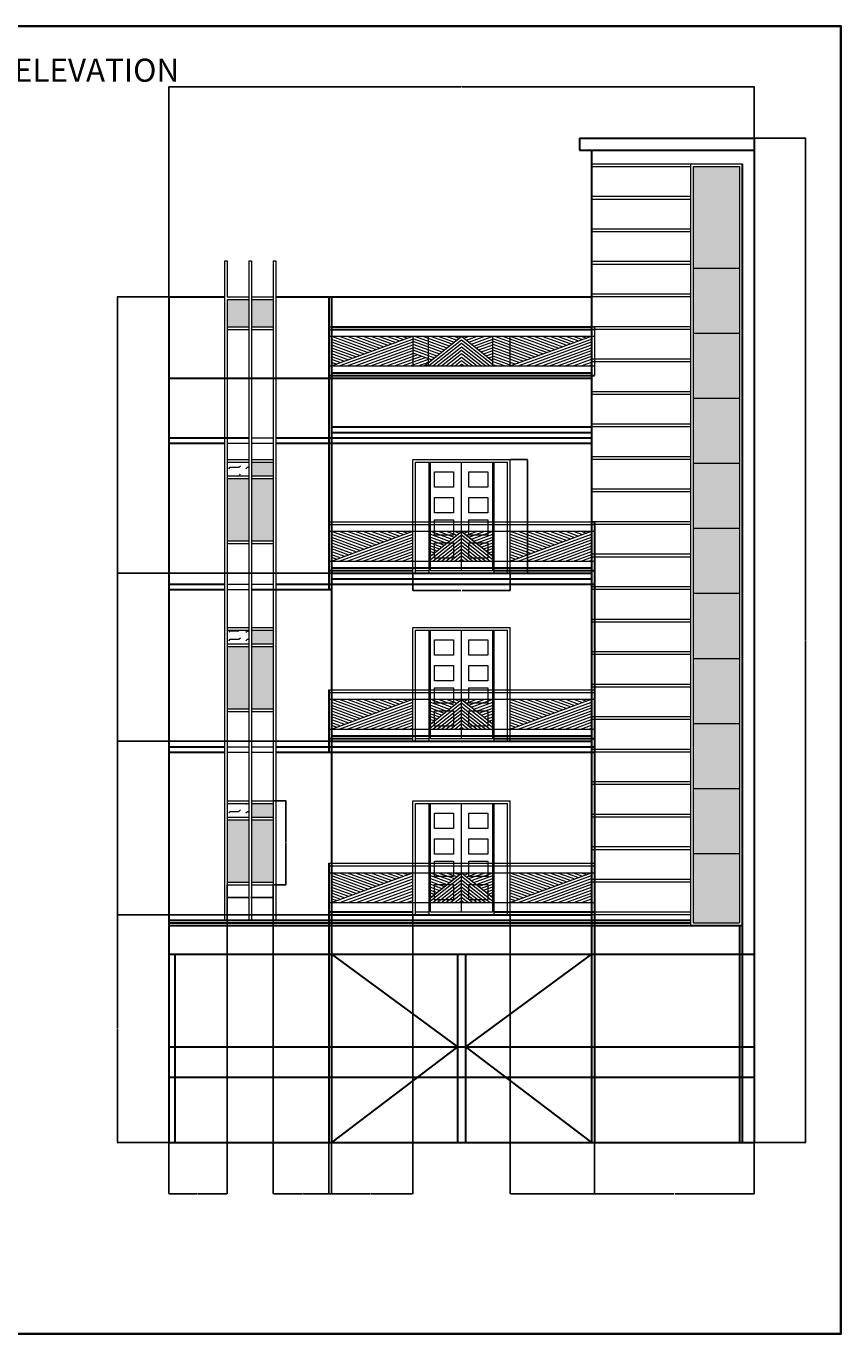
# Model space of a CAD drawing. Units: inches. Extents: x 2220 to 3422, y 783 to 1748.
# Tile 7 of 7: x 2821 to 3422, y 783 to 1748. Entities that reach past the tile are written whole.
import ezdxf

# ---------------------------------------------------------------- set-up
doc = ezdxf.new("R2010")
doc.units = ezdxf.units.IN
for name, color, linetype, lineweight in [('A-ANNO-DIMS', 2, 'Continuous', 18), ('A-ANNO-TEXT', 7, 'Continuous', 30), ('A-ANNO-TTLB', 7, 'Continuous', 35), ('A-ELEV', 7, 'Continuous', 30), ('A-ELEV-CLAD', 8, 'Continuous', 18), ('A-ELEV-DOOR', 3, 'Continuous', 20), ('A-ELEV-GLAZ', 4, 'Continuous', 18), ('A-ELEV-PATT', 252, 'Continuous', 13), ('A-ELEV-RAIL', 7, 'Continuous', 20)]:
    doc.layers.add(name, color=color, linetype=linetype, lineweight=lineweight)
doc.styles.get("Standard").update_dxf_attribs({"font": 'arial.ttf'})
doc.dimstyles.get("Standard").update_dxf_attribs({"dimtxt": 0.18, "dimasz": 0.18, "dimexe": 0.18, "dimexo": 0.0625, "dimgap": 0.09, "dimtad": 0, "dimtih": 1, "dimtoh": 1, "dimdec": 4, "dimzin": 0, "dimdsep": 46, "dimtxsty": 'Standard', "dimcen": 0.09, "dimadec": 0, "dimazin": 0, "dimtfac": 1, "dimtdec": 4, "dimtofl": 0, "dimtmove": 0, "dimatfit": 3, "dimfxl": 1, "dimtolj": 1, "dimtzin": 0, "dimarcsym": 0})

# ---------------------------------------------------------------- blocks, each defined once
blk = doc.blocks.new('DOOR-ELEV-DOUBLE-PANELED')
for p, q in [((0, 0), (0, 84)), ((0, 84), (72, 84)), ((2, 0), (2, 82)), ((2, 82), (70, 82)), ((12, 0), (12, 82)), ((13, 2), (13, 82)), ((36, 2), (36, 82)), ((59, 2), (59, 82)), ((60, 0), (60, 82)), ((70, 0), (70, 82)), ((72, 0), (72, 84)), ((2, 2), (12, 2)), ((13, 2), (59, 2))]:
    blk.add_line(p, q)
for points in [[(16.01, 74.85), (30.01, 74.85), (30.01, 63.54), (16.01, 63.54)], [(41.44, 74.85), (55.44, 74.85), (55.44, 63.54), (41.44, 63.54)], [(16.01, 55.98), (30.01, 55.98), (30.01, 44.68), (16.01, 44.68)], [(41.44, 55.98), (55.44, 55.98), (55.44, 44.68), (41.44, 44.68)], [(16.01, 39.54), (30.01, 39.54), (30.01, 28.24), (16.01, 28.24)], [(41.44, 39.54), (55.44, 39.54), (55.44, 28.24), (41.44, 28.24)], [(16.01, 22.35), (30.01, 22.35), (30.01, 11.05), (16.01, 11.05)], [(41.44, 22.35), (55.44, 22.35), (55.44, 11.05), (41.44, 11.05)]]:
    blk.add_lwpolyline(points, close=True)
blk = doc.blocks.new('GLAZ-ELEV-PAIRED-LIGHTS')
for p, q in [((0, 62), (16, 62)), ((0, 60), (16, 60)), ((0, 60), (0, 50)), ((18, 62), (34, 62)), ((18, 60), (34, 60)), ((34, 60), (34, 50)), ((0, 50), (16, 50)), ((18, 50), (34, 50)), ((0, 48), (16, 48)), ((0, 48), (0, 2)), ((18, 48), (34, 48)), ((34, 48), (34, 2)), ((0, 2), (16, 2)), ((0, 0), (16, 0)), ((18, 2), (34, 2)), ((18, 0), (34, 0))]:
    blk.add_line(p, q)
blk = doc.blocks.new('*D33')
at = {"layer": 'A-ANNO-DIMS', "color": 0, "lineweight": -2, "transparency": 16777216}
for p, q in [((3178.51, 1428.15), (3191.23, 1428.15)), ((3191.05, 1427.97), (3191.05, 1386.33)), ((3191.05, 1344.33), (3191.05, 1385.97)), ((3178.51, 1344.15), (3191.23, 1344.15))]:
    blk.add_line(p, q, dxfattribs=at)
at = {"layer": 'A-ANNO-DIMS', "color": 0, "transparency": 16777216}
for points in [[(3191.02, 1427.97), (3191.08, 1427.97), (3191.05, 1428.15)], [(3191.02, 1344.33), (3191.08, 1344.33), (3191.05, 1344.15)]]:
    blk.add_solid(points, dxfattribs=at)
at = {"layer": 'Defpoints', "color": 0, "transparency": 16777216}
for p in [(3178.45, 1428.15), (3191.05, 1428.15), (3178.45, 1344.15)]:
    blk.add_point(p, dxfattribs=at)
at = {"layer": 'A-ANNO-DIMS', "color": 0, "transparency": 16777216, "insert": (3191.05, 1386.15), "char_height": 0.18, "attachment_point": 5}
blk.add_mtext('\\A1;DOUBLE DOOR 84 TYP.', dxfattribs=at)
blk = doc.blocks.new('*D34')
at = {"layer": 'A-ANNO-DIMS', "color": 0, "lineweight": -2, "transparency": 16777216}
for p, q in [((3106.45, 1344.09), (3106.45, 1331.37)), ((3178.45, 1344.09), (3178.45, 1331.37)), ((3106.63, 1331.55), (3141.92, 1331.55)), ((3178.27, 1331.55), (3142.97, 1331.55))]:
    blk.add_line(p, q, dxfattribs=at)
at = {"layer": 'A-ANNO-DIMS', "color": 0, "transparency": 16777216}
for points in [[(3106.63, 1331.58), (3106.63, 1331.52), (3106.45, 1331.55)], [(3178.27, 1331.58), (3178.27, 1331.52), (3178.45, 1331.55)]]:
    blk.add_solid(points, dxfattribs=at)
at = {"layer": 'Defpoints', "color": 0, "transparency": 16777216}
for p in [(3106.45, 1344.15), (3178.45, 1344.15), (3178.45, 1331.55)]:
    blk.add_point(p, dxfattribs=at)
at = {"layer": 'A-ANNO-DIMS', "color": 0, "transparency": 16777216, "insert": (3142.45, 1331.55), "char_height": 0.18, "attachment_point": 5}
blk.add_mtext('\\A1;72 TYP.', dxfattribs=at)
blk = doc.blocks.new('*D35')
at = {"layer": 'A-ANNO-DIMS', "color": 0, "lineweight": -2, "transparency": 16777216}
for p, q in [((3003.51, 1176.15), (3012.93, 1176.15)), ((3012.75, 1175.97), (3012.75, 1145.33)), ((3012.75, 1114.33), (3012.75, 1144.97)), ((3003.51, 1114.15), (3012.93, 1114.15))]:
    blk.add_line(p, q, dxfattribs=at)
at = {"layer": 'A-ANNO-DIMS', "color": 0, "transparency": 16777216}
for points in [[(3012.72, 1175.97), (3012.78, 1175.97), (3012.75, 1176.15)], [(3012.72, 1114.33), (3012.78, 1114.33), (3012.75, 1114.15)]]:
    blk.add_solid(points, dxfattribs=at)
at = {"layer": 'Defpoints', "color": 0, "transparency": 16777216}
for p in [(3003.45, 1176.15), (3012.75, 1176.15), (3003.45, 1114.15)]:
    blk.add_point(p, dxfattribs=at)
at = {"layer": 'A-ANNO-DIMS', "color": 0, "transparency": 16777216, "insert": (3012.75, 1145.15), "char_height": 0.18, "attachment_point": 5}
blk.add_mtext('\\A1;PAIRED LIGHTS 62 TYP.', dxfattribs=at)
blk = doc.blocks.new('*D36')
at = {"layer": 'A-ANNO-DIMS', "color": 0, "lineweight": -2, "transparency": 16777216}
for p, q in [((2969.45, 1114.09), (2969.45, 1104.67)), ((3003.45, 1114.09), (3003.45, 1104.67)), ((2969.63, 1104.85), (2985.92, 1104.85)), ((3003.27, 1104.85), (2986.97, 1104.85))]:
    blk.add_line(p, q, dxfattribs=at)
at = {"layer": 'A-ANNO-DIMS', "color": 0, "transparency": 16777216}
for points in [[(2969.63, 1104.88), (2969.63, 1104.82), (2969.45, 1104.85)], [(3003.27, 1104.88), (3003.27, 1104.82), (3003.45, 1104.85)]]:
    blk.add_solid(points, dxfattribs=at)
at = {"layer": 'Defpoints', "color": 0, "transparency": 16777216}
for p in [(2969.45, 1114.15), (3003.45, 1114.15), (3003.45, 1104.85)]:
    blk.add_point(p, dxfattribs=at)
at = {"layer": 'A-ANNO-DIMS', "color": 0, "transparency": 16777216, "insert": (2986.45, 1104.85), "char_height": 0.18, "attachment_point": 5}
blk.add_mtext('\\A1;34 TYP.', dxfattribs=at)
blk = doc.blocks.new('*D61')
at = {"layer": 'A-ANNO-DIMS', "color": 0, "lineweight": -2, "transparency": 16777216}
for p, q in [((2926.45, 1548.21), (2926.45, 1703.46)), ((2926.63, 1703.28), (3142.15, 1703.28)), ((3358.27, 1703.28), (3142.74, 1703.28)), ((3358.45, 1665.44), (3358.45, 1703.46))]:
    blk.add_line(p, q, dxfattribs=at)
at = {"layer": 'A-ANNO-DIMS', "color": 0, "transparency": 16777216}
for points in [[(2926.63, 1703.31), (2926.63, 1703.25), (2926.45, 1703.28)], [(3358.27, 1703.31), (3358.27, 1703.25), (3358.45, 1703.28)]]:
    blk.add_solid(points, dxfattribs=at)
at = {"layer": 'Defpoints', "color": 0, "transparency": 16777216}
for p in [(3358.45, 1703.28), (3358.45, 1665.38), (2926.45, 1548.15)]:
    blk.add_point(p, dxfattribs=at)
at = {"layer": 'A-ANNO-DIMS', "color": 0, "transparency": 16777216, "insert": (3142.45, 1703.28), "char_height": 0.18, "attachment_point": 5}
blk.add_mtext('\\A1;432', dxfattribs=at)
blk = doc.blocks.new('*D62')
at = {"layer": 'A-ANNO-DIMS', "color": 0, "lineweight": -2, "transparency": 16777216}
for p, q in [((3358.51, 1665.38), (3396.53, 1665.38)), ((3396.35, 1665.2), (3396.35, 1294.94)), ((3396.35, 924.33), (3396.35, 1294.58)), ((3358.51, 924.15), (3396.53, 924.15))]:
    blk.add_line(p, q, dxfattribs=at)
at = {"layer": 'A-ANNO-DIMS', "color": 0, "transparency": 16777216}
for points in [[(3396.32, 1665.2), (3396.38, 1665.2), (3396.35, 1665.38)], [(3396.32, 924.33), (3396.38, 924.33), (3396.35, 924.15)]]:
    blk.add_solid(points, dxfattribs=at)
at = {"layer": 'Defpoints', "color": 0, "transparency": 16777216}
for p in [(3358.45, 1665.38), (3396.35, 1665.38), (3358.45, 924.15)]:
    blk.add_point(p, dxfattribs=at)
at = {"layer": 'A-ANNO-DIMS', "color": 0, "transparency": 16777216, "insert": (3396.35, 1294.76), "char_height": 0.18, "attachment_point": 5}
blk.add_mtext('\\A1;741.2', dxfattribs=at)
blk = doc.blocks.new('*D63')
at = {"layer": 'A-ANNO-DIMS', "color": 0, "lineweight": -2, "transparency": 16777216}
for p, q in [((2969.45, 1114.09), (2969.45, 886.07)), ((2926.45, 1088.09), (2926.45, 886.07)), ((2926.63, 886.25), (2947.72, 886.25)), ((2969.27, 886.25), (2948.17, 886.25))]:
    blk.add_line(p, q, dxfattribs=at)
at = {"layer": 'A-ANNO-DIMS', "color": 0, "transparency": 16777216}
for points in [[(2926.63, 886.28), (2926.63, 886.22), (2926.45, 886.25)], [(2969.27, 886.28), (2969.27, 886.22), (2969.45, 886.25)]]:
    blk.add_solid(points, dxfattribs=at)
at = {"layer": 'Defpoints', "color": 0, "transparency": 16777216}
for p in [(2969.45, 1114.15), (2926.45, 1088.15), (2969.45, 886.25)]:
    blk.add_point(p, dxfattribs=at)
at = {"layer": 'A-ANNO-DIMS', "color": 0, "transparency": 16777216, "insert": (2947.95, 886.25), "char_height": 0.18, "attachment_point": 5}
blk.add_mtext('\\A1;43', dxfattribs=at)
blk = doc.blocks.new('*D64')
at = {"layer": 'A-ANNO-DIMS', "color": 0, "lineweight": -2, "transparency": 16777216}
for p, q in [((3003.45, 1114.09), (3003.45, 886.07)), ((3046.45, 1092.09), (3046.45, 886.07)), ((3003.63, 886.25), (3024.72, 886.25)), ((3046.27, 886.25), (3025.17, 886.25))]:
    blk.add_line(p, q, dxfattribs=at)
at = {"layer": 'A-ANNO-DIMS', "color": 0, "transparency": 16777216}
for points in [[(3003.63, 886.28), (3003.63, 886.22), (3003.45, 886.25)], [(3046.27, 886.28), (3046.27, 886.22), (3046.45, 886.25)]]:
    blk.add_solid(points, dxfattribs=at)
at = {"layer": 'Defpoints', "color": 0, "transparency": 16777216}
for p in [(3003.45, 1114.15), (3046.45, 1092.15), (3046.45, 886.25)]:
    blk.add_point(p, dxfattribs=at)
at = {"layer": 'A-ANNO-DIMS', "color": 0, "transparency": 16777216, "insert": (3024.95, 886.25), "char_height": 0.18, "attachment_point": 5}
blk.add_mtext('\\A1;43', dxfattribs=at)
blk = doc.blocks.new('*D65')
at = {"layer": 'A-ANNO-DIMS', "color": 0, "lineweight": -2, "transparency": 16777216}
for p, q in [((3106.45, 1092.09), (3106.45, 886.07)), ((3044.45, 924.09), (3044.45, 886.07)), ((3044.63, 886.25), (3075.23, 886.25)), ((3106.27, 886.25), (3075.66, 886.25))]:
    blk.add_line(p, q, dxfattribs=at)
at = {"layer": 'A-ANNO-DIMS', "color": 0, "transparency": 16777216}
for points in [[(3044.63, 886.28), (3044.63, 886.22), (3044.45, 886.25)], [(3106.27, 886.28), (3106.27, 886.22), (3106.45, 886.25)]]:
    blk.add_solid(points, dxfattribs=at)
at = {"layer": 'Defpoints', "color": 0, "transparency": 16777216}
for p in [(3106.45, 1092.15), (3044.45, 924.15), (3106.45, 886.25)]:
    blk.add_point(p, dxfattribs=at)
at = {"layer": 'A-ANNO-DIMS', "color": 0, "transparency": 16777216, "insert": (3075.45, 886.25), "char_height": 0.18, "attachment_point": 5}
blk.add_mtext('\\A1;62', dxfattribs=at)
blk = doc.blocks.new('*D66')
at = {"layer": 'A-ANNO-DIMS', "color": 0, "lineweight": -2, "transparency": 16777216}
for p, q in [((3178.45, 1092.09), (3178.45, 886.07)), ((3240.45, 924.09), (3240.45, 886.07)), ((3178.63, 886.25), (3209.23, 886.25)), ((3240.27, 886.25), (3209.66, 886.25))]:
    blk.add_line(p, q, dxfattribs=at)
at = {"layer": 'A-ANNO-DIMS', "color": 0, "transparency": 16777216}
for points in [[(3178.63, 886.28), (3178.63, 886.22), (3178.45, 886.25)], [(3240.27, 886.28), (3240.27, 886.22), (3240.45, 886.25)]]:
    blk.add_solid(points, dxfattribs=at)
at = {"layer": 'Defpoints', "color": 0, "transparency": 16777216}
for p in [(3178.45, 1092.15), (3240.45, 924.15), (3240.45, 886.25)]:
    blk.add_point(p, dxfattribs=at)
at = {"layer": 'A-ANNO-DIMS', "color": 0, "transparency": 16777216, "insert": (3209.45, 886.25), "char_height": 0.18, "attachment_point": 5}
blk.add_mtext('\\A1;62', dxfattribs=at)
blk = doc.blocks.new('*D67')
at = {"layer": 'A-ANNO-DIMS', "color": 0, "lineweight": -2, "transparency": 16777216}
for p, q in [((3240.45, 924.09), (3240.45, 886.07)), ((3358.45, 924.09), (3358.45, 886.07)), ((3240.63, 886.25), (3299.17, 886.25)), ((3358.27, 886.25), (3299.73, 886.25))]:
    blk.add_line(p, q, dxfattribs=at)
at = {"layer": 'A-ANNO-DIMS', "color": 0, "transparency": 16777216}
for points in [[(3240.63, 886.28), (3240.63, 886.22), (3240.45, 886.25)], [(3358.27, 886.28), (3358.27, 886.22), (3358.45, 886.25)]]:
    blk.add_solid(points, dxfattribs=at)
at = {"layer": 'Defpoints', "color": 0, "transparency": 16777216}
for p in [(3240.45, 924.15), (3358.45, 924.15), (3358.45, 886.25)]:
    blk.add_point(p, dxfattribs=at)
at = {"layer": 'A-ANNO-DIMS', "color": 0, "transparency": 16777216, "insert": (3299.45, 886.25), "char_height": 0.18, "attachment_point": 5}
blk.add_mtext('\\A1;118', dxfattribs=at)
blk = doc.blocks.new('*D68')
at = {"layer": 'A-ANNO-DIMS', "color": 0, "lineweight": -2, "transparency": 16777216}
for p, q in [((3106.38, 1092.15), (2888.37, 1092.15)), ((2888.55, 1091.97), (2888.55, 1008.33)), ((2888.55, 924.33), (2888.55, 1007.97)), ((2926.38, 924.15), (2888.37, 924.15))]:
    blk.add_line(p, q, dxfattribs=at)
at = {"layer": 'A-ANNO-DIMS', "color": 0, "transparency": 16777216}
for points in [[(2888.52, 1091.97), (2888.58, 1091.97), (2888.55, 1092.15)], [(2888.52, 924.33), (2888.58, 924.33), (2888.55, 924.15)]]:
    blk.add_solid(points, dxfattribs=at)
at = {"layer": 'Defpoints', "color": 0, "transparency": 16777216}
for p in [(3106.45, 1092.15), (2888.55, 924.15), (2926.45, 924.15)]:
    blk.add_point(p, dxfattribs=at)
at = {"layer": 'A-ANNO-DIMS', "color": 0, "transparency": 16777216, "insert": (2888.55, 1008.15), "char_height": 0.18, "attachment_point": 5}
blk.add_mtext('\\A1;168', dxfattribs=at)
blk = doc.blocks.new('*D69')
at = {"layer": 'A-ANNO-DIMS', "color": 0, "lineweight": -2, "transparency": 16777216}
for p, q in [((3106.38, 1220.15), (2888.37, 1220.15)), ((2888.55, 1219.97), (2888.55, 1156.33)), ((2888.55, 1092.33), (2888.55, 1155.97)), ((3106.38, 1092.15), (2888.37, 1092.15))]:
    blk.add_line(p, q, dxfattribs=at)
at = {"layer": 'A-ANNO-DIMS', "color": 0, "transparency": 16777216}
for points in [[(2888.52, 1219.97), (2888.58, 1219.97), (2888.55, 1220.15)], [(2888.52, 1092.33), (2888.58, 1092.33), (2888.55, 1092.15)]]:
    blk.add_solid(points, dxfattribs=at)
at = {"layer": 'Defpoints', "color": 0, "transparency": 16777216}
for p in [(2888.55, 1220.15), (3106.45, 1220.15), (3106.45, 1092.15)]:
    blk.add_point(p, dxfattribs=at)
at = {"layer": 'A-ANNO-DIMS', "color": 0, "transparency": 16777216, "insert": (2888.55, 1156.15), "char_height": 0.18, "attachment_point": 5}
blk.add_mtext('\\A1;128', dxfattribs=at)
blk = doc.blocks.new('*D70')
at = {"layer": 'A-ANNO-DIMS', "color": 0, "lineweight": -2, "transparency": 16777216}
for p, q in [((3106.38, 1344.15), (2888.37, 1344.15)), ((2888.55, 1343.97), (2888.55, 1282.33)), ((2888.55, 1220.33), (2888.55, 1281.97)), ((3106.38, 1220.15), (2888.37, 1220.15))]:
    blk.add_line(p, q, dxfattribs=at)
at = {"layer": 'A-ANNO-DIMS', "color": 0, "transparency": 16777216}
for points in [[(2888.52, 1343.97), (2888.58, 1343.97), (2888.55, 1344.15)], [(2888.52, 1220.33), (2888.58, 1220.33), (2888.55, 1220.15)]]:
    blk.add_solid(points, dxfattribs=at)
at = {"layer": 'Defpoints', "color": 0, "transparency": 16777216}
for p in [(2888.55, 1344.15), (3106.45, 1344.15), (3106.45, 1220.15)]:
    blk.add_point(p, dxfattribs=at)
at = {"layer": 'A-ANNO-DIMS', "color": 0, "transparency": 16777216, "insert": (2888.55, 1282.15), "char_height": 0.18, "attachment_point": 5}
blk.add_mtext('\\A1;124', dxfattribs=at)
blk = doc.blocks.new('*D71')
at = {"layer": 'A-ANNO-DIMS', "color": 0, "lineweight": -2, "transparency": 16777216}
for p, q in [((2926.38, 1548.15), (2888.37, 1548.15)), ((2888.55, 1547.97), (2888.55, 1446.33)), ((2888.55, 1344.33), (2888.55, 1445.97)), ((3106.38, 1344.15), (2888.37, 1344.15))]:
    blk.add_line(p, q, dxfattribs=at)
at = {"layer": 'A-ANNO-DIMS', "color": 0, "transparency": 16777216}
for points in [[(2888.52, 1547.97), (2888.58, 1547.97), (2888.55, 1548.15)], [(2888.52, 1344.33), (2888.58, 1344.33), (2888.55, 1344.15)]]:
    blk.add_solid(points, dxfattribs=at)
at = {"layer": 'Defpoints', "color": 0, "transparency": 16777216}
for p in [(2926.45, 1548.15), (2888.55, 1344.15), (3106.45, 1344.15)]:
    blk.add_point(p, dxfattribs=at)
at = {"layer": 'A-ANNO-DIMS', "color": 0, "transparency": 16777216, "insert": (2888.55, 1446.15), "char_height": 0.18, "attachment_point": 5}
blk.add_mtext('\\A1;204', dxfattribs=at)

msp = doc.modelspace()

# ---------------------------------------------------------------- hatches: boundary and pattern name
at = {"layer": 'A-ELEV-PATT'}
h = msp.add_hatch(dxfattribs=at)
h.set_pattern_fill('GOST_GLASS', color=256)
h.paths.add_polyline_path([(3347.4457, 1644.3759), (3313.4457, 1644.3759), (3313.4457, 1569.3627), (3347.4457, 1569.3627)])
h.paths.add_polyline_path([(3347.4457, 1569.3627), (3313.4457, 1569.3627), (3313.4457, 1521.3627), (3347.4457, 1521.3627)])
h.paths.add_polyline_path([(3347.4457, 1521.3627), (3313.4457, 1521.3627), (3313.4457, 1473.3627), (3347.4457, 1473.3627)])
h.paths.add_polyline_path([(3347.4457, 1473.3627), (3313.4457, 1473.3627), (3313.4457, 1425.3627), (3347.4457, 1425.3627)])
h.paths.add_polyline_path([(3347.4457, 1425.3627), (3313.4457, 1425.3627), (3313.4457, 1377.3627), (3347.4457, 1377.3627)])
h.paths.add_polyline_path([(3347.4457, 1377.3627), (3313.4457, 1377.3627), (3313.4457, 1329.3627), (3347.4457, 1329.3627)])
h.paths.add_polyline_path([(3347.4457, 1329.3627), (3313.4457, 1329.3627), (3313.4457, 1281.3627), (3347.4457, 1281.3627)])
h.paths.add_polyline_path([(3347.4457, 1281.3627), (3313.4457, 1281.3627), (3313.4457, 1233.3627), (3347.4457, 1233.3627)])
h.paths.add_polyline_path([(3347.4457, 1233.3627), (3313.4457, 1233.3627), (3313.4457, 1185.3627), (3347.4457, 1185.3627)])
h.paths.add_polyline_path([(3347.4457, 1185.3627), (3313.4457, 1185.3627), (3313.4457, 1137.3627), (3347.4457, 1137.3627)])
h.paths.add_polyline_path([(3347.4457, 1137.3627), (3313.4457, 1137.3627), (3313.4457, 1086.1482), (3347.4457, 1086.1482)])
h.paths.add_polyline_path([(2985.4457, 1546.1482), (2969.4457, 1546.1482), (2969.4457, 1526.1482), (2985.4457, 1526.1482)])
h.paths.add_polyline_path([(3003.4457, 1546.1482), (2987.4457, 1546.1482), (2987.4457, 1526.1482), (3003.4457, 1526.1482)])
h.paths.add_polyline_path([(3003.4457, 1414.1482), (2987.4457, 1414.1482), (2987.4457, 1368.1482), (3003.4457, 1368.1482)])
h.paths.add_polyline_path([(2985.4457, 1414.1482), (2969.4457, 1414.1482), (2969.4457, 1368.1482), (2985.4457, 1368.1482)])
h.paths.add_polyline_path([(3003.4457, 1426.1482), (2987.4457, 1426.1482), (2987.4457, 1416.1482), (3003.4457, 1416.1482)])
h.paths.add_polyline_path([(2985.4457, 1290.1482), (2969.4457, 1290.1482), (2969.4457, 1244.1482), (2985.4457, 1244.1482)])
h.paths.add_polyline_path([(3003.4457, 1302.1482), (2987.4457, 1302.1482), (2987.4457, 1292.1482), (3003.4457, 1292.1482)])
h.paths.add_polyline_path([(3003.4457, 1290.1482), (2987.4457, 1290.1482), (2987.4457, 1244.1482), (3003.4457, 1244.1482)])
h.paths.add_polyline_path([(2985.4457, 1162.1482), (2969.4457, 1162.1482), (2969.4457, 1116.1482), (2985.4457, 1116.1482)])
h.paths.add_polyline_path([(3003.4457, 1162.1482), (2987.4457, 1162.1482), (2987.4457, 1116.1482), (3003.4457, 1116.1482)])
h.paths.add_polyline_path([(3003.4457, 1174.1482), (2987.4457, 1174.1482), (2987.4457, 1164.1482), (3003.4457, 1164.1482)])
h = msp.add_hatch(dxfattribs=at)
h.set_pattern_fill('ANSI31', color=256, scale=0.631485, angle=-24.8637, style=0)
h.paths.add_polyline_path([(3046.4457, 1497.1482), (3118.0937, 1497.1482), (3118.0937, 1502.6032), (3106.4457, 1506.8732), (3106.4457, 1519.1482)])
h = msp.add_hatch(dxfattribs=at)
h.set_pattern_fill('ANSI31', color=256, scale=0.6296784, angle=114.8637, style=0)
h.paths.add_polyline_path([(3046.4457, 1497.1482), (3106.4457, 1519.1482), (3046.4457, 1519.1482)])
h = msp.add_hatch(dxfattribs=at)
h.set_pattern_fill('ANSI31', color=256, scale=0.6299657, angle=114.8637, style=0)
h.paths.add_polyline_path([(3106.4457, 1506.8732), (3120.5927, 1501.6862), (3142.4457, 1519.1482), (3106.4457, 1519.1482)])
h = msp.add_hatch(dxfattribs=at)
h.set_pattern_fill('ANSI31', color=256, scale=0.63046, angle=-6.54629, style=0)
h.paths.add_polyline_path([(3114.8777, 1497.1482), (3142.4457, 1497.1482), (3142.4457, 1519.1482)])
h = msp.add_hatch(dxfattribs=at)
h.set_pattern_fill('ANSI31', color=256, scale=0.6298828, angle=96.54629, style=0)
h.paths.add_polyline_path([(3142.4457, 1497.1482), (3165.4457, 1497.1482), (3165.4457, 1500.7752), (3142.4457, 1519.1482)])
h = msp.add_hatch(dxfattribs=at)
h.set_pattern_fill('ANSI31', color=256, scale=0.630929, angle=-24.8637, style=0)
h.paths.add_polyline_path([(3142.4457, 1519.1482), (3165.4457, 1500.7752), (3165.4457, 1519.1482)])
h = msp.add_hatch(dxfattribs=at)
h.set_pattern_fill('ANSI31', color=256, scale=0.6300432, angle=114.8637, style=0)
h.paths.add_polyline_path([(3165.4457, 1497.1482), (3178.4457, 1497.1482), (3238.4457, 1519.1482), (3165.4457, 1519.1482)])
h = msp.add_hatch(dxfattribs=at)
h.set_pattern_fill('ANSI31', color=256, scale=0.628795, angle=-24.8637, style=0)
h.paths.add_polyline_path([(3178.4457, 1497.1482), (3238.4457, 1497.1482), (3238.4457, 1519.1482)])
h = msp.add_hatch(dxfattribs=at)
h.set_pattern_fill('FLEX', color=256)
h.paths.add_polyline_path([(2985.4457, 1174.1482), (2969.4457, 1174.1482), (2969.4457, 1164.1482), (2985.4457, 1164.1482)])
h.paths.add_polyline_path([(2985.4457, 1302.1482), (2969.4457, 1302.1482), (2969.4457, 1292.1482), (2985.4457, 1292.1482)])
h.paths.add_polyline_path([(2985.4457, 1426.1482), (2969.4457, 1426.1482), (2969.4457, 1416.1482), (2985.4457, 1416.1482)])
h = msp.add_hatch(dxfattribs=at)
h.set_pattern_fill('ANSI31', color=256, scale=0.6290295, angle=-24.8637, style=0)
h.paths.add_polyline_path([(3046.4457, 1353.1482), (3106.4457, 1353.1482), (3106.4457, 1375.1482)])
h = msp.add_hatch(dxfattribs=at)
h.set_pattern_fill('ANSI31', color=256, scale=0.6298801, angle=114.8637, style=0)
h.paths.add_polyline_path([(3046.4457, 1353.1482), (3106.4457, 1375.1482), (3046.4457, 1375.1482)])
h = msp.add_hatch(dxfattribs=at)
h.set_pattern_fill('ANSI31', color=256, scale=0.6295074, angle=-6.546291, style=0)
h.paths.add_polyline_path([(3118.0937, 1353.1482), (3142.4457, 1353.1482), (3142.4457, 1375.1482), (3118.4457, 1355.9812), (3118.4457, 1353.4282)])
h = msp.add_hatch(dxfattribs=at)
h.set_pattern_fill('ANSI31', color=256, scale=0.630182, angle=114.8637, style=0)
h.paths.add_polyline_path([(3119.4457, 1356.7752), (3142.4457, 1375.1482), (3119.4457, 1375.1482)])
h = msp.add_hatch(dxfattribs=at)
h.set_pattern_fill('ANSI31', color=256, scale=0.629722, angle=96.5463, style=0)
h.paths.add_polyline_path([(3142.4457, 1353.1482), (3165.4457, 1353.1482), (3165.4457, 1356.7752), (3142.4457, 1375.1482)])
h = msp.add_hatch(dxfattribs=at)
h.set_pattern_fill('ANSI31', color=256, scale=0.627861, angle=-24.8637, style=0)
h.paths.add_polyline_path([(3142.4457, 1375.1482), (3165.4457, 1356.7752), (3165.4457, 1375.1482)])
h = msp.add_hatch(dxfattribs=at)
h.set_pattern_fill('ANSI31', color=256, scale=0.630795, angle=-24.8637, style=0)
h.paths.add_polyline_path([(3178.4457, 1353.1482), (3238.4457, 1353.1482), (3238.4457, 1375.1482)])
h = msp.add_hatch(dxfattribs=at)
h.set_pattern_fill('ANSI31', color=256, scale=0.6297335, angle=114.8637, style=0)
h.paths.add_polyline_path([(3178.4457, 1353.1482), (3238.4457, 1375.1482), (3178.4457, 1375.1482)])
h = msp.add_hatch(dxfattribs=at)
h.set_pattern_fill('ANSI31', color=256, scale=0.625554, angle=-24.8637, style=0)
h.paths.add_polyline_path([(3046.4457, 1229.1482), (3106.4457, 1229.1482), (3106.4457, 1251.1482)])
h = msp.add_hatch(dxfattribs=at)
h.set_pattern_fill('ANSI31', color=256, scale=0.6297588, angle=114.8637, style=0)
h.paths.add_polyline_path([(3046.4457, 1229.1482), (3106.4457, 1251.1482), (3046.4457, 1251.1482)])
h = msp.add_hatch(dxfattribs=at)
h.set_pattern_fill('ANSI31', color=256, scale=0.630262, angle=-6.54629, style=0)
h.paths.add_polyline_path([(3118.0937, 1229.1482), (3142.4457, 1229.1482), (3142.4457, 1251.1482), (3118.4457, 1231.9812), (3118.4457, 1229.4282)])
h = msp.add_hatch(dxfattribs=at)
h.set_pattern_fill('ANSI31', color=256, scale=0.6300775, angle=114.8637, style=0)
h.paths.add_polyline_path([(3119.4457, 1232.7752), (3142.4457, 1251.1482), (3119.4457, 1251.1482)])
h = msp.add_hatch(dxfattribs=at)
h.set_pattern_fill('ANSI31', color=256, scale=0.629907, angle=96.5463, style=0)
h.paths.add_polyline_path([(3142.4457, 1229.1482), (3165.4457, 1229.1482), (3165.4457, 1232.7752), (3142.4457, 1251.1482)])
h = msp.add_hatch(dxfattribs=at)
h.set_pattern_fill('ANSI31', color=256, scale=0.63681, angle=-24.8637, style=0)
h.paths.add_polyline_path([(3142.4457, 1251.1482), (3165.4457, 1232.7752), (3165.4457, 1251.1482)])
h = msp.add_hatch(dxfattribs=at)
h.set_pattern_fill('ANSI31', color=256, scale=0.628068, angle=-24.8637, style=0)
h.paths.add_polyline_path([(3178.4457, 1229.1482), (3238.4457, 1229.1482), (3238.4457, 1251.1482)])
h = msp.add_hatch(dxfattribs=at)
h.set_pattern_fill('ANSI31', color=256, scale=0.6301624, angle=114.8637, style=0)
h.paths.add_polyline_path([(3178.4457, 1229.1482), (3238.4457, 1251.1482), (3178.4457, 1251.1482)])
h = msp.add_hatch(dxfattribs=at)
h.set_pattern_fill('ANSI31', color=256, scale=0.6709154, angle=-24.8637, style=0)
h.paths.add_polyline_path([(3046.4457, 1101.1482), (3106.4457, 1101.1482), (3106.4457, 1123.1482)])
h = msp.add_hatch(dxfattribs=at)
h.set_pattern_fill('ANSI31', color=256, scale=0.6296968, angle=114.8637, style=0)
h.paths.add_polyline_path([(3046.4457, 1101.1482), (3106.4457, 1123.1482), (3046.4457, 1123.1482)])
h = msp.add_hatch(dxfattribs=at)
h.set_pattern_fill('ANSI31', color=256, scale=0.6303695, angle=-6.546291, style=0)
h.paths.add_polyline_path([(3118.0937, 1101.1482), (3142.4457, 1101.1482), (3142.4457, 1123.1482), (3118.4457, 1103.9812), (3118.4457, 1101.4282)])
h = msp.add_hatch(dxfattribs=at)
h.set_pattern_fill('ANSI31', color=256, scale=0.6300341, angle=114.8637, style=0)
h.paths.add_polyline_path([(3119.4457, 1104.7752), (3142.4457, 1123.1482), (3119.4457, 1123.1482)])
h = msp.add_hatch(dxfattribs=at)
h.set_pattern_fill('ANSI31', color=256, scale=0.6298537, angle=96.54629, style=0)
h.paths.add_polyline_path([(3142.4457, 1101.1482), (3165.4457, 1101.1482), (3165.4457, 1104.7752), (3142.4457, 1123.1482)])
h = msp.add_hatch(dxfattribs=at)
h.set_pattern_fill('ANSI31', color=256, scale=0.6169294, angle=-24.8637, style=0)
h.paths.add_polyline_path([(3142.4457, 1123.1482), (3165.4457, 1104.7752), (3165.4457, 1123.1482)])
h = msp.add_hatch(dxfattribs=at)
h.set_pattern_fill('ANSI31', color=256, scale=0.633624, angle=-24.8637, style=0)
h.paths.add_polyline_path([(3178.4457, 1101.1482), (3238.4457, 1101.1482), (3238.4457, 1123.1482)])
h = msp.add_hatch(dxfattribs=at)
h.set_pattern_fill('ANSI31', color=256, scale=0.6301242, angle=114.8637, style=0)
h.paths.add_polyline_path([(3178.4457, 1101.1482), (3238.4457, 1123.1482), (3178.4457, 1123.1482)])

# ---------------------------------------------------------------- linework, layer by layer
at = {"layer": 'A-ANNO-TTLB'}
msp.add_lwpolyline([(2220.0037, 1747.9465), (3422.343, 1747.9465), (3422.343, 782.804), (2220.0037, 782.804)], close=True, dxfattribs=at)
at = {"layer": 'A-ELEV'}
for p, q in [((3229.4457, 1665.3759), (3358.4457, 1665.3759)), ((3229.4457, 1665.3759), (3229.4457, 1656.3759)), ((3358.4457, 1665.3759), (3358.4457, 1656.3759)), ((3229.4457, 1656.3759), (3358.4457, 1656.3759)), ((3238.4457, 1656.3759), (3238.4457, 924.1482)), ((3358.4457, 1656.3759), (3358.4457, 924.1482)), ((3349.4457, 1646.3759), (3349.4457, 924.1482)), ((2926.4457, 1548.1482), (2967.4457, 1548.1482)), ((2926.4457, 1548.1482), (2926.4457, 924.1482)), ((3005.4457, 1548.1482), (3238.4457, 1548.1482)), ((3044.4457, 1548.1482), (3044.4457, 1340.1482)), ((3046.4457, 1548.1482), (3046.4457, 1340.1482)), ((3046.4457, 1526.1482), (3238.4457, 1526.1482)), ((3046.4457, 1524.1482), (3238.4457, 1524.1482)), ((2926.4457, 1488.1482), (3238.4457, 1488.1482)), ((3044.4457, 1490.1482), (3106.4457, 1490.1482)), ((3046.4457, 1492.1482), (3238.4457, 1492.1482)), ((3046.4457, 1488.1482), (3238.4457, 1488.1482)), ((3046.4457, 1488.1482), (3238.4457, 1488.1482)), ((3046.4457, 1488.1482), (3238.4457, 1488.1482)), ((3106.4457, 1490.1482), (3119.4457, 1490.1482)), ((3119.4457, 1490.1482), (3166.4457, 1490.1482)), ((3166.4457, 1490.1482), (3240.4457, 1490.1482)), ((3046.4457, 1452.1482), (3238.4457, 1452.1482)), ((3046.4457, 1448.1482), (3238.4457, 1448.1482)), ((2926.4457, 1444.1482), (2985.4457, 1444.1482)), ((2926.4457, 1440.1482), (2967.4457, 1440.1482)), ((3005.4457, 1444.1482), (3238.4457, 1444.1482)), ((3005.4457, 1440.1482), (3238.4457, 1440.1482)), ((3044.4457, 1382.1482), (3044.4457, 1336.1482)), ((3240.4457, 1382.1482), (3240.4457, 1336.1482)), ((3240.4457, 1382.1482), (3240.4457, 1084.1482)), ((3044.4457, 1346.1482), (3106.4457, 1346.1482)), ((3046.4457, 1348.1482), (3238.4457, 1348.1482)), ((3046.4457, 1344.1482), (3238.4457, 1344.1482)), ((3046.4457, 1344.1482), (3238.4457, 1344.1482)), ((3046.4457, 1344.1482), (3238.4457, 1344.1482)), ((3166.4457, 1346.1482), (3240.4457, 1346.1482)), ((2926.4457, 1336.1482), (2967.4457, 1336.1482)), ((2926.4457, 1332.1482), (2967.4457, 1332.1482)), ((2987.4457, 1332.1482), (3046.4457, 1332.1482)), ((3005.4457, 1336.1482), (3240.4457, 1336.1482)), ((3044.4457, 1340.1482), (3044.4457, 1332.1482)), ((3046.4457, 1340.1482), (3238.4457, 1340.1482)), ((3046.4457, 1340.1482), (3046.4457, 924.1482)), ((3044.4457, 1258.1482), (3044.4457, 1212.1482)), ((3240.4457, 1258.1482), (3240.4457, 1212.1482)), ((2926.4457, 1216.1482), (2967.4457, 1216.1482)), ((3005.4457, 1216.1482), (3240.4457, 1216.1482)), ((3044.4457, 1222.1482), (3106.4457, 1222.1482)), ((3046.4457, 1224.1482), (3238.4457, 1224.1482)), ((3046.4457, 1220.1482), (3238.4457, 1220.1482)), ((3046.4457, 1220.1482), (3238.4457, 1220.1482)), ((3166.4457, 1222.1482), (3240.4457, 1222.1482)), ((2926.4457, 1212.1482), (2967.4457, 1212.1482)), ((3005.4457, 1212.1482), (3240.4457, 1212.1482)), ((3044.4457, 1130.1482), (3044.4457, 924.1482)), ((3044.4457, 1130.1482), (3044.4457, 924.1482)), ((3240.4457, 1130.1482), (3240.4457, 924.1482)), ((3044.4457, 1094.1482), (3106.4457, 1094.1482)), ((3046.4457, 1092.1482), (3238.4457, 1092.1482)), ((3166.4457, 1094.1482), (3240.4457, 1094.1482)), ((2926.4457, 1088.1482), (3311.4457, 1088.1482)), ((2926.4457, 1086.1482), (3311.4457, 1086.1482)), ((2926.4457, 1084.1482), (3349.4457, 1084.1482)), ((3347.4457, 1084.1482), (3347.4457, 924.1482)), ((2926.4457, 1063.0824), (3358.4457, 1063.0824)), ((2930.9143, 1063.0824), (2930.9143, 924.1482)), ((3046.4457, 1063.0824), (3139.4457, 994.5824)), ((3139.4457, 1063.0824), (3139.4457, 924.1482)), ((3145.4457, 1063.0824), (3145.4457, 924.1482)), ((3238.4457, 1063.0824), (3145.4457, 994.5824)), ((2926.4457, 994.5824), (3358.4457, 994.5824)), ((3139.4457, 994.5824), (3046.4457, 924.1482)), ((3145.4457, 994.5824), (3238.4457, 924.1482)), ((2926.4457, 972.1482), (3358.4457, 972.1482)), ((2926.4457, 924.1482), (3358.4457, 924.1482))]:
    msp.add_line(p, q, dxfattribs=at)
at = {"layer": 'A-ELEV-CLAD'}
for p, q in [((3238.4457, 1646.3759), (3311.4457, 1646.3759)), ((3238.4457, 1644.3759), (3311.4457, 1644.3759)), ((3262.4457, 1646.3759), (3335.4457, 1646.3759)), ((3262.4457, 1644.3759), (3311.4457, 1644.3759)), ((3311.4457, 1646.3759), (3311.4457, 1084.1482)), ((3311.4457, 1646.3759), (3349.4457, 1646.3759)), ((3238.4457, 1622.3759), (3311.4457, 1622.3759)), ((3238.4457, 1620.3759), (3311.4457, 1620.3759)), ((3238.4457, 1598.3759), (3311.4457, 1598.3759)), ((3238.4457, 1596.3759), (3311.4457, 1596.3759)), ((3238.4457, 1574.3759), (3311.4457, 1574.3759)), ((3238.4457, 1572.3759), (3311.4457, 1572.3759)), ((3238.4457, 1550.3759), (3311.4457, 1550.3759)), ((3238.4457, 1548.3759), (3311.4457, 1548.3759)), ((3238.4457, 1526.3759), (3311.4457, 1526.3759)), ((3238.4457, 1524.3759), (3311.4457, 1524.3759)), ((3238.4457, 1502.3759), (3311.4457, 1502.3759)), ((3238.4457, 1500.3759), (3311.4457, 1500.3759)), ((3238.4457, 1478.3759), (3311.4457, 1478.3759)), ((3238.4457, 1476.3759), (3311.4457, 1476.3759)), ((3238.4457, 1454.3759), (3311.4457, 1454.3759)), ((3238.4457, 1452.3759), (3311.4457, 1452.3759)), ((3238.4457, 1430.3759), (3311.4457, 1430.3759)), ((3238.4457, 1428.3759), (3311.4457, 1428.3759)), ((3238.4457, 1406.3759), (3311.4457, 1406.3759)), ((3238.4457, 1404.3759), (3311.4457, 1404.3759)), ((3238.4457, 1382.3759), (3311.4457, 1382.3759)), ((3238.4457, 1380.3759), (3311.4457, 1380.3759)), ((3238.4457, 1358.3759), (3311.4457, 1358.3759)), ((3238.4457, 1356.3759), (3311.4457, 1356.3759)), ((3238.4457, 1334.3759), (3311.4457, 1334.3759)), ((3238.4457, 1332.3759), (3311.4457, 1332.3759)), ((3238.4457, 1310.3759), (3311.4457, 1310.3759)), ((3238.4457, 1308.3759), (3311.4457, 1308.3759)), ((3238.4457, 1286.3759), (3311.4457, 1286.3759)), ((3238.4457, 1284.3759), (3311.4457, 1284.3759)), ((3238.4457, 1262.3759), (3311.4457, 1262.3759)), ((3238.4457, 1260.3759), (3311.4457, 1260.3759)), ((3238.4457, 1238.3759), (3311.4457, 1238.3759)), ((3238.4457, 1236.3759), (3311.4457, 1236.3759)), ((3238.4457, 1214.3759), (3311.4457, 1214.3759)), ((3238.4457, 1212.3759), (3311.4457, 1212.3759)), ((3238.4457, 1190.3759), (3311.4457, 1190.3759)), ((3238.4457, 1188.3759), (3311.4457, 1188.3759)), ((3238.4457, 1166.3759), (3311.4457, 1166.3759)), ((3238.4457, 1164.3759), (3311.4457, 1164.3759)), ((3238.4457, 1142.3759), (3311.4457, 1142.3759)), ((3238.4457, 1140.3759), (3311.4457, 1140.3759)), ((3238.4457, 1118.3759), (3311.4457, 1118.3759)), ((3238.4457, 1116.3759), (3311.4457, 1116.3759)), ((3238.4457, 1094.3759), (3311.4457, 1094.3759)), ((3238.4457, 1092.3759), (3311.4457, 1092.3759))]:
    msp.add_line(p, q, dxfattribs=at)
at = {"layer": 'A-ELEV-GLAZ'}
for p, q in [((3313.4457, 1644.3759), (3313.4457, 1086.1482)), ((3313.4457, 1644.3759), (3347.4457, 1644.3759)), ((3313.4457, 1644.3759), (3347.4457, 1644.3759)), ((3347.4457, 1644.3759), (3347.4457, 1086.1482)), ((2967.4457, 1574.6715), (2967.4457, 1088.1482)), ((2967.4457, 1574.6715), (2969.4457, 1574.6715)), ((2969.4457, 1574.6715), (2969.4457, 1548.1482)), ((2985.4457, 1574.6715), (2985.4457, 1088.1482)), ((2985.4457, 1574.6715), (2987.4457, 1574.6715)), ((2987.4457, 1574.6715), (2987.4457, 1116.1482)), ((3003.4457, 1574.6715), (3003.4457, 1088.1482)), ((3003.4457, 1574.6715), (3005.4457, 1574.6715)), ((3005.4457, 1574.6715), (3005.4457, 1088.1482)), ((3313.4457, 1569.3627), (3347.4457, 1569.3627)), ((2969.4457, 1548.1482), (2985.4457, 1548.1482)), ((2969.4457, 1546.1482), (2985.4457, 1546.1482)), ((2969.4457, 1546.1482), (2969.4457, 1088.1482)), ((2987.4457, 1548.1482), (3003.4457, 1548.1482)), ((2987.4457, 1546.1482), (3003.4457, 1546.1482)), ((2969.4457, 1526.1482), (2985.4457, 1526.1482)), ((2987.4457, 1526.1482), (3003.4457, 1526.1482)), ((2969.4457, 1524.1482), (2985.4457, 1524.1482)), ((2987.4457, 1524.1482), (3003.4457, 1524.1482)), ((3313.4457, 1521.3627), (3347.4457, 1521.3627)), ((3313.4457, 1473.3627), (3347.4457, 1473.3627)), ((2969.4457, 1440.1482), (2985.4457, 1440.1482)), ((2987.4457, 1444.1482), (3003.4457, 1444.1482)), ((2987.4457, 1440.1482), (3003.4457, 1440.1482)), ((3313.4457, 1425.3627), (3347.4457, 1425.3627)), ((3313.4457, 1377.3627), (3347.4457, 1377.3627)), ((2969.4457, 1336.1482), (2985.4457, 1336.1482)), ((2969.4457, 1332.1482), (2985.4457, 1332.1482)), ((2987.4457, 1336.1482), (3003.4457, 1336.1482)), ((3313.4457, 1329.3627), (3347.4457, 1329.3627)), ((3313.4457, 1281.3627), (3347.4457, 1281.3627)), ((3313.4457, 1233.3627), (3347.4457, 1233.3627)), ((2969.4457, 1216.1482), (2985.4457, 1216.1482)), ((2987.4457, 1216.1482), (3003.4457, 1216.1482)), ((2969.4457, 1212.1482), (2985.4457, 1212.1482)), ((2987.4457, 1212.1482), (3003.4457, 1212.1482)), ((3313.4457, 1185.3627), (3347.4457, 1185.3627)), ((2987.4457, 1176.1482), (2987.4457, 1088.1482)), ((3313.4457, 1137.3627), (3347.4457, 1137.3627)), ((3313.4457, 1086.1482), (3347.4457, 1086.1482))]:
    msp.add_line(p, q, dxfattribs=at)
at = {"layer": 'A-ELEV-RAIL'}
for p, q in [((3044.4457, 1526.1482), (3240.4457, 1526.1482)), ((3240.4457, 1526.1482), (3240.4457, 1490.1482)), ((3044.4457, 1524.1482), (3240.4457, 1524.1482)), ((3044.4457, 1519.1482), (3240.4457, 1519.1482)), ((3046.4457, 1497.1482), (3106.4457, 1519.1482)), ((3106.4457, 1519.1482), (3106.4457, 1497.1482)), ((3114.8777, 1497.1482), (3142.5815, 1519.1482)), ((3118.0938, 1497.1482), (3118.0938, 1519.1482)), ((3142.3099, 1519.1482), (3165.4457, 1500.7757)), ((3165.4457, 1497.1482), (3165.4457, 1519.1105)), ((3178.4457, 1497.1482), (3238.4457, 1519.1482)), ((3178.4457, 1497.1482), (3178.4457, 1519.1482)), ((3044.3801, 1513.515), (3044.4457, 1513.4909)), ((3044.4457, 1497.1482), (3240.4457, 1497.1482)), ((3044.4457, 1382.1482), (3240.4457, 1382.1482)), ((3044.4457, 1380.1482), (3240.4457, 1380.1482)), ((3044.4457, 1375.1482), (3240.4457, 1375.1482)), ((3046.4457, 1353.1482), (3106.4457, 1375.1482)), ((3118.4457, 1355.9816), (3142.5815, 1375.1482)), ((3142.3099, 1375.1482), (3165.4457, 1356.7757)), ((3178.4457, 1353.1482), (3238.4457, 1375.1482)), ((3044.3801, 1369.515), (3044.4457, 1369.4909)), ((3108.4457, 1369.4909), (3108.5112, 1369.515)), ((3044.4457, 1353.1482), (3240.4457, 1353.1482)), ((3044.4457, 1258.1482), (3240.4457, 1258.1482)), ((3044.4457, 1256.1482), (3240.4457, 1256.1482)), ((3044.3801, 1245.515), (3044.4457, 1245.4909)), ((3044.4457, 1251.1482), (3240.4457, 1251.1482)), ((3046.4457, 1229.1482), (3106.4457, 1251.1482)), ((3108.4457, 1245.4909), (3108.5112, 1245.515)), ((3118.4457, 1231.9816), (3142.5815, 1251.1482)), ((3142.3099, 1251.1482), (3165.4457, 1232.7757)), ((3178.4457, 1229.1482), (3238.4457, 1251.1482)), ((3044.4457, 1229.1482), (3240.4457, 1229.1482)), ((3044.4457, 1130.1482), (3240.4457, 1130.1482)), ((3044.4457, 1128.1482), (3240.4457, 1128.1482)), ((3044.4457, 1123.1482), (3240.4457, 1123.1482)), ((3046.4457, 1101.1482), (3106.4457, 1123.1482)), ((3118.4457, 1103.9816), (3142.5815, 1123.1482)), ((3142.3099, 1123.1482), (3165.4457, 1104.7757)), ((3178.4457, 1101.1482), (3238.4457, 1123.1482)), ((3044.3801, 1117.515), (3044.4457, 1117.4909)), ((3108.4457, 1117.4909), (3108.5112, 1117.515)), ((3044.4457, 1101.1482), (3240.4457, 1101.1482))]:
    msp.add_line(p, q, dxfattribs=at)

# ---------------------------------------------------------------- block references
at = {"layer": 'A-ELEV-DOOR'}
for p in [(3106.446, 1344.148), (3106.446, 1220.148), (3106.446, 1092.148)]:
    msp.add_blockref('DOOR-ELEV-DOUBLE-PANELED', p, dxfattribs=at)
at = {"layer": 'A-ELEV-GLAZ'}
for p in [(2969.446, 1366.148), (2969.446, 1242.148), (2969.446, 1114.148)]:
    msp.add_blockref('GLAZ-ELEV-PAIRED-LIGHTS', p, dxfattribs=at)

# ---------------------------------------------------------------- texts
at = {"layer": 'A-ANNO-TEXT'}
msp.add_text('PLAN AND ELEVATION', height=17, dxfattribs=at).set_placement((2696.7314, 1706.9332))

# ---------------------------------------------------------------- dimensions: what is measured, and where the dimension line sits
at = {"layer": 'A-ANNO-DIMS'}
for base, p1, p2, picture, middle in [((3358.4457, 1703.2759), (2926.4457, 1548.1482), (3358.4457, 1665.3759), '*D61', (3142.4457, 1703.2759)), ((2969.4457, 886.2482), (2926.4457, 1088.1482), (2969.4457, 1114.1482), '*D63', (2947.9457, 886.2482)), ((3046.4457, 886.2482), (3003.4457, 1114.1482), (3046.4457, 1092.1482), '*D64', (3024.9457, 886.2482)), ((3106.4457, 886.2482), (3044.4457, 924.1482), (3106.4457, 1092.1482), '*D65', (3075.4457, 886.2482)), ((3240.4457, 886.2482), (3178.4457, 1092.1482), (3240.4457, 924.1482), '*D66', (3209.4457, 886.2482)), ((3358.4457, 886.2482), (3240.4457, 924.1482), (3358.4457, 924.1482), '*D67', (3299.4457, 886.2482))]:
    dim = msp.add_linear_dim(base=base, p1=p1, p2=p2, dimstyle='Standard', override={"dimdec": 0, "dimlfac": 1, "dimrnd": 0, "dimzin": 0, "dimdsep": 46, "dimlunit": 2}, dxfattribs=at)
    dim.commit()
    dim.dimension.update_dxf_attribs({"geometry": picture, "text_midpoint": middle})
for base, p1, p2, override, picture, middle in [((3396.3457, 1665.3759), (3358.4457, 924.1482), (3358.4457, 1665.3759), {"dimdec": 1, "dimlfac": 1, "dimrnd": 0, "dimzin": 0, "dimdsep": 46, "dimlunit": 2}, '*D62', (3396.3457, 1294.762)), ((2888.5457, 1344.1482), (2926.4457, 1548.1482), (3106.4457, 1344.1482), {"dimdec": 0, "dimlfac": 1, "dimrnd": 0, "dimzin": 0, "dimdsep": 46, "dimlunit": 2}, '*D71', (2888.5457, 1446.1482)), ((2888.5457, 1344.1482), (3106.4457, 1220.1482), (3106.4457, 1344.1482), {"dimdec": 0, "dimlfac": 1, "dimrnd": 0, "dimzin": 0, "dimdsep": 46, "dimlunit": 2}, '*D70', (2888.5457, 1282.1482)), ((2888.5457, 1220.1482), (3106.4457, 1092.1482), (3106.4457, 1220.1482), {"dimdec": 0, "dimlfac": 1, "dimrnd": 0, "dimzin": 0, "dimdsep": 46, "dimlunit": 2}, '*D69', (2888.5457, 1156.1482)), ((2888.5457, 924.1482), (3106.4457, 1092.1482), (2926.4457, 924.1482), {"dimdec": 0, "dimlfac": 1, "dimrnd": 0, "dimzin": 0, "dimdsep": 46, "dimlunit": 2}, '*D68', (2888.5457, 1008.1482))]:
    dim = msp.add_linear_dim(base=base, p1=p1, p2=p2, angle=90, dimstyle='Standard', override=override, dxfattribs=at)
    dim.commit()
    dim.dimension.update_dxf_attribs({"geometry": picture, "text_midpoint": middle})
for base, p1, p2, text, picture, middle in [((3191.0457, 1428.1482), (3178.4457, 1344.1482), (3178.4457, 1428.1482), 'DOUBLE DOOR <> TYP.', '*D33', (3191.0457, 1386.1482)), ((3012.7457, 1176.1482), (3003.4457, 1114.1482), (3003.4457, 1176.1482), 'PAIRED LIGHTS <> TYP.', '*D35', (3012.7457, 1145.1482))]:
    dim = msp.add_linear_dim(base=base, p1=p1, p2=p2, angle=90, text=text, dimstyle='Standard', override={"dimdec": 0, "dimlfac": 1, "dimrnd": 0, "dimzin": 0, "dimdsep": 46, "dimlunit": 2}, dxfattribs=at)
    dim.commit()
    dim.dimension.update_dxf_attribs({"geometry": picture, "text_midpoint": middle})
for base, p1, p2, picture, middle in [((3178.4457, 1331.5482), (3106.4457, 1344.1482), (3178.4457, 1344.1482), '*D34', (3142.4457, 1331.5482)), ((3003.4457, 1104.8482), (2969.4457, 1114.1482), (3003.4457, 1114.1482), '*D36', (2986.4457, 1104.8482))]:
    dim = msp.add_linear_dim(base=base, p1=p1, p2=p2, text='<> TYP.', dimstyle='Standard', override={"dimdec": 0, "dimlfac": 1, "dimrnd": 0, "dimzin": 0, "dimdsep": 46, "dimlunit": 2}, dxfattribs=at)
    dim.commit()
    dim.dimension.update_dxf_attribs({"geometry": picture, "text_midpoint": middle})

doc.saveas('drawing.dxf')
